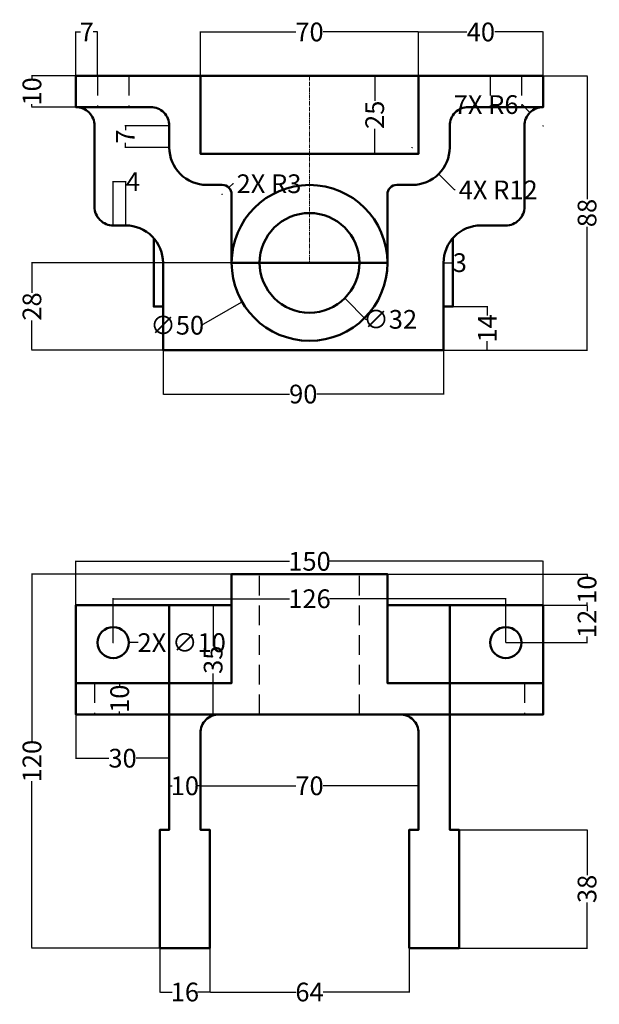
# Model space of a CAD drawing. Units: millimetres. Extents: x 17 to 203, y -197 to 119.
import ezdxf

# ---------------------------------------------------------------- set-up
doc = ezdxf.new("R2010")
doc.units = ezdxf.units.MM
doc.header["$MEASUREMENT"] = 0
doc.linetypes.add('CENTER', pattern=[2, 1.25, -0.25, 0.25, -0.25])
doc.linetypes.add('HIDDEN', pattern=[9.525, 6.35, -3.175])
for name, color, linetype, lineweight in [('M-CNTR', 4, 'CENTER', 18), ('M-CONS', 8, 'Continuous', 13), ('M-DIMS', 2, 'Continuous', 18), ('M-HIDN', 3, 'HIDDEN', 25), ('M-OUTL', 7, 'Continuous', 50)]:
    doc.layers.add(name, color=color, linetype=linetype, lineweight=lineweight)
doc.styles.get("Standard").update_dxf_attribs({"font": 'arial.ttf'})
doc.dimstyles.get("Standard").update_dxf_attribs({"dimtxt": 6, "dimasz": 0.18, "dimexe": 0.18, "dimexo": 0.0625, "dimgap": 0.09, "dimtad": 0, "dimtoh": 1, "dimdec": 0, "dimzin": 0, "dimdsep": 46, "dimtxsty": 'Standard', "dimcen": 0.09, "dimadec": 0, "dimazin": 0, "dimtfac": 1, "dimtdec": 0, "dimtofl": 0, "dimtmove": 0, "dimatfit": 3, "dimfxl": 1, "dimtolj": 1, "dimtzin": 0, "dimarcsym": 0})

# ---------------------------------------------------------------- blocks, each defined once
blk = doc.blocks.new('MOUNT-HOLE-D10')
blk.add_circle((0, 0), 5)
blk = doc.blocks.new('MOUNT-HOLE-D10-EDGE')
for p, q in [((-5, 10), (-5, 0)), ((5, 10), (5, 0))]:
    blk.add_line(p, q)
blk = doc.blocks.new('*D3')
at = {"layer": 'Defpoints', "color": 0, "transparency": 16777216}
for p in [(184.66, -55.03), (34.66, -69.11), (184.66, -69.11)]:
    blk.add_point(p, dxfattribs=at)
at = {"layer": 'M-DIMS', "color": 0, "lineweight": -2, "transparency": 16777216}
for p, q in [((34.66, -69.05), (34.66, -54.85)), ((34.84, -55.03), (103.23, -55.03)), ((184.48, -55.03), (116.08, -55.03)), ((184.66, -69.05), (184.66, -54.85))]:
    blk.add_line(p, q, dxfattribs=at)
at = {"layer": 'M-DIMS', "color": 0, "transparency": 16777216}
for points in [[(34.84, -55), (34.84, -55.06), (34.66, -55.03)], [(184.48, -55), (184.48, -55.06), (184.66, -55.03)]]:
    blk.add_solid(points, dxfattribs=at)
at = {"layer": 'M-DIMS', "color": 0, "transparency": 16777216, "insert": (109.66, -55.03), "char_height": 6, "attachment_point": 5}
blk.add_mtext('\\A1;150', dxfattribs=at)
blk = doc.blocks.new('*D4')
at = {"layer": 'Defpoints', "color": 0, "transparency": 16777216}
for p in [(41.66, 114.77), (34.66, 100.7), (41.66, 100.7)]:
    blk.add_point(p, dxfattribs=at)
at = {"layer": 'M-DIMS', "color": 0, "lineweight": -2, "transparency": 16777216}
for p, q in [((34.66, 100.76), (34.66, 114.95)), ((34.84, 114.77), (36.13, 114.77)), ((41.48, 114.77), (40.19, 114.77)), ((41.66, 100.76), (41.66, 114.95))]:
    blk.add_line(p, q, dxfattribs=at)
at = {"layer": 'M-DIMS', "color": 0, "transparency": 16777216}
for points in [[(34.84, 114.8), (34.84, 114.74), (34.66, 114.77)], [(41.48, 114.8), (41.48, 114.74), (41.66, 114.77)]]:
    blk.add_solid(points, dxfattribs=at)
at = {"layer": 'M-DIMS', "color": 0, "transparency": 16777216, "insert": (38.16, 114.77), "char_height": 6, "attachment_point": 5}
blk.add_mtext('\\A1;7', dxfattribs=at)
blk = doc.blocks.new('*D5')
at = {"layer": 'Defpoints', "color": 0, "transparency": 16777216}
for p in [(144.66, 114.77), (74.66, 100.7), (144.66, 100.7)]:
    blk.add_point(p, dxfattribs=at)
at = {"layer": 'M-DIMS', "color": 0, "lineweight": -2, "transparency": 16777216}
for p, q in [((74.66, 100.76), (74.66, 114.95)), ((74.84, 114.77), (105.31, 114.77)), ((144.48, 114.77), (114.01, 114.77)), ((144.66, 100.76), (144.66, 114.95))]:
    blk.add_line(p, q, dxfattribs=at)
at = {"layer": 'M-DIMS', "color": 0, "transparency": 16777216}
for points in [[(74.84, 114.8), (74.84, 114.74), (74.66, 114.77)], [(144.48, 114.8), (144.48, 114.74), (144.66, 114.77)]]:
    blk.add_solid(points, dxfattribs=at)
at = {"layer": 'M-DIMS', "color": 0, "transparency": 16777216, "insert": (109.66, 114.77), "char_height": 6, "attachment_point": 5}
blk.add_mtext('\\A1;70', dxfattribs=at)
blk = doc.blocks.new('*D6')
at = {"layer": 'Defpoints', "color": 0, "transparency": 16777216}
for p in [(184.66, 114.77), (144.66, 100.7), (184.66, 100.7)]:
    blk.add_point(p, dxfattribs=at)
at = {"layer": 'M-DIMS', "color": 0, "lineweight": -2, "transparency": 16777216}
for p, q in [((144.66, 100.76), (144.66, 114.95)), ((144.84, 114.77), (160.16, 114.77)), ((184.48, 114.77), (169.16, 114.77)), ((184.66, 100.76), (184.66, 114.95))]:
    blk.add_line(p, q, dxfattribs=at)
at = {"layer": 'M-DIMS', "color": 0, "transparency": 16777216}
for points in [[(144.84, 114.8), (144.84, 114.74), (144.66, 114.77)], [(184.48, 114.8), (184.48, 114.74), (184.66, 114.77)]]:
    blk.add_solid(points, dxfattribs=at)
at = {"layer": 'M-DIMS', "color": 0, "transparency": 16777216, "insert": (164.66, 114.77), "char_height": 6, "attachment_point": 5}
blk.add_mtext('\\A1;40', dxfattribs=at)
blk = doc.blocks.new('*D7')
at = {"layer": 'Defpoints', "color": 0, "transparency": 16777216}
for p in [(184.66, 100.7), (152.66, 12.7), (198.73, 12.7)]:
    blk.add_point(p, dxfattribs=at)
at = {"layer": 'M-DIMS', "color": 0, "lineweight": -2, "transparency": 16777216}
for p, q in [((184.72, 100.7), (198.91, 100.7)), ((198.73, 100.52), (198.73, 61.09)), ((198.73, 12.88), (198.73, 52.3)), ((152.72, 12.7), (198.91, 12.7))]:
    blk.add_line(p, q, dxfattribs=at)
at = {"layer": 'M-DIMS', "color": 0, "transparency": 16777216}
for points in [[(198.7, 100.52), (198.76, 100.52), (198.73, 100.7)], [(198.7, 12.88), (198.76, 12.88), (198.73, 12.7)]]:
    blk.add_solid(points, dxfattribs=at)
at = {"layer": 'M-DIMS', "color": 0, "transparency": 16777216, "insert": (198.73, 56.7), "char_height": 6, "attachment_point": 5, "rotation": 90}
blk.add_mtext('\\A1;88', dxfattribs=at)
blk = doc.blocks.new('*D8')
at = {"layer": 'Defpoints', "color": 0, "transparency": 16777216}
for p in [(34.66, 100.7), (20.58, 90.7), (34.66, 90.7)]:
    blk.add_point(p, dxfattribs=at)
at = {"layer": 'M-DIMS', "color": 0, "lineweight": -2, "transparency": 16777216}
for p, q in [((34.6, 100.7), (20.4, 100.7)), ((20.58, 100.52), (20.58, 99.79)), ((20.58, 90.88), (20.58, 91.6)), ((34.6, 90.7), (20.4, 90.7))]:
    blk.add_line(p, q, dxfattribs=at)
at = {"layer": 'M-DIMS', "color": 0, "transparency": 16777216}
for points in [[(20.55, 100.52), (20.61, 100.52), (20.58, 100.7)], [(20.55, 90.88), (20.61, 90.88), (20.58, 90.7)]]:
    blk.add_solid(points, dxfattribs=at)
at = {"layer": 'M-DIMS', "color": 0, "transparency": 16777216, "insert": (20.58, 95.7), "char_height": 6, "attachment_point": 5, "rotation": 90}
blk.add_mtext('\\A1;10', dxfattribs=at)
blk = doc.blocks.new('*D9')
at = {"layer": 'Defpoints', "color": 0, "transparency": 16777216}
for p in [(130.58, 100.7), (144.66, 100.7), (144.66, 75.7)]:
    blk.add_point(p, dxfattribs=at)
at = {"layer": 'M-DIMS', "color": 0, "lineweight": -2, "transparency": 16777216}
for p, q in [((144.6, 100.7), (130.4, 100.7)), ((130.58, 100.52), (130.58, 92.66)), ((130.58, 75.88), (130.58, 83.74)), ((144.6, 75.7), (130.4, 75.7))]:
    blk.add_line(p, q, dxfattribs=at)
at = {"layer": 'M-DIMS', "color": 0, "transparency": 16777216}
for points in [[(130.55, 100.52), (130.61, 100.52), (130.58, 100.7)], [(130.55, 75.88), (130.61, 75.88), (130.58, 75.7)]]:
    blk.add_solid(points, dxfattribs=at)
at = {"layer": 'M-DIMS', "color": 0, "transparency": 16777216, "insert": (130.58, 88.2), "char_height": 6, "attachment_point": 5, "rotation": 90}
blk.add_mtext('\\A1;25', dxfattribs=at)
blk = doc.blocks.new('*D10')
at = {"layer": 'Defpoints', "color": 0, "transparency": 16777216}
for p in [(20.58, 40.7), (84.66, 40.7), (62.66, 12.7)]:
    blk.add_point(p, dxfattribs=at)
at = {"layer": 'M-DIMS', "color": 0, "lineweight": -2, "transparency": 16777216}
for p, q in [((84.6, 40.7), (20.4, 40.7)), ((20.58, 40.52), (20.58, 31.14)), ((20.58, 12.88), (20.58, 22.25)), ((62.6, 12.7), (20.4, 12.7))]:
    blk.add_line(p, q, dxfattribs=at)
at = {"layer": 'M-DIMS', "color": 0, "transparency": 16777216}
for points in [[(20.55, 40.52), (20.61, 40.52), (20.58, 40.7)], [(20.55, 12.88), (20.61, 12.88), (20.58, 12.7)]]:
    blk.add_solid(points, dxfattribs=at)
at = {"layer": 'M-DIMS', "color": 0, "transparency": 16777216, "insert": (20.58, 26.7), "char_height": 6, "attachment_point": 5, "rotation": 90}
blk.add_mtext('\\A1;28', dxfattribs=at)
blk = doc.blocks.new('*D11')
at = {"layer": 'Defpoints', "color": 0, "transparency": 16777216}
for p in [(62.66, 12.7), (152.66, 12.7), (62.66, -1.38)]:
    blk.add_point(p, dxfattribs=at)
at = {"layer": 'M-DIMS', "color": 0, "lineweight": -2, "transparency": 16777216}
for p, q in [((62.66, 12.63), (62.66, -1.56)), ((152.66, 12.63), (152.66, -1.56)), ((62.84, -1.38), (103.28, -1.38)), ((152.48, -1.38), (112.04, -1.38))]:
    blk.add_line(p, q, dxfattribs=at)
at = {"layer": 'M-DIMS', "color": 0, "transparency": 16777216}
for points in [[(62.84, -1.35), (62.84, -1.41), (62.66, -1.38)], [(152.48, -1.35), (152.48, -1.41), (152.66, -1.38)]]:
    blk.add_solid(points, dxfattribs=at)
at = {"layer": 'M-DIMS', "color": 0, "transparency": 16777216, "insert": (107.66, -1.38), "char_height": 6, "attachment_point": 5}
blk.add_mtext('\\A1;90', dxfattribs=at)
blk = doc.blocks.new('*D12')
at = {"layer": 'Defpoints', "color": 0, "transparency": 16777216}
for p in [(152.66, 26.7), (152.66, 12.7), (166.73, 12.7)]:
    blk.add_point(p, dxfattribs=at)
at = {"layer": 'M-DIMS', "color": 0, "lineweight": -2, "transparency": 16777216}
for p, q in [((152.72, 26.7), (166.91, 26.7)), ((166.73, 26.52), (166.73, 23.79)), ((152.72, 12.7), (166.91, 12.7)), ((166.73, 12.88), (166.73, 15.6))]:
    blk.add_line(p, q, dxfattribs=at)
at = {"layer": 'M-DIMS', "color": 0, "transparency": 16777216}
for points in [[(166.7, 26.52), (166.76, 26.52), (166.73, 26.7)], [(166.7, 12.88), (166.76, 12.88), (166.73, 12.7)]]:
    blk.add_solid(points, dxfattribs=at)
at = {"layer": 'M-DIMS', "color": 0, "transparency": 16777216, "insert": (166.73, 19.7), "char_height": 6, "attachment_point": 5, "rotation": 90}
blk.add_mtext('\\A1;14', dxfattribs=at)
blk = doc.blocks.new('*D13')
at = {"layer": 'Defpoints', "color": 0, "transparency": 16777216}
for p in [(155.66, 40.77), (152.66, 26.7), (155.66, 26.7)]:
    blk.add_point(p, dxfattribs=at)
at = {"layer": 'M-DIMS', "color": 0, "lineweight": -2, "transparency": 16777216}
for p, q in [((152.66, 26.76), (152.66, 40.95)), ((152.84, 40.77), (155.48, 40.77)), ((155.66, 26.76), (155.66, 40.95)), ((155.66, 40.77), (155.84, 40.77))]:
    blk.add_line(p, q, dxfattribs=at)
at = {"layer": 'M-DIMS', "color": 0, "transparency": 16777216}
for points in [[(152.84, 40.8), (152.84, 40.74), (152.66, 40.77)], [(155.48, 40.8), (155.48, 40.74), (155.66, 40.77)]]:
    blk.add_solid(points, dxfattribs=at)
at = {"layer": 'M-DIMS', "color": 0, "transparency": 16777216, "insert": (157.89, 40.77), "char_height": 6, "attachment_point": 5}
blk.add_mtext('\\A1;3', dxfattribs=at)
blk = doc.blocks.new('*D14')
at = {"layer": 'Defpoints', "color": 0, "transparency": 16777216}
for p in [(50.66, 66.77), (46.66, 52.7), (50.66, 52.7)]:
    blk.add_point(p, dxfattribs=at)
at = {"layer": 'M-DIMS', "color": 0, "lineweight": -2, "transparency": 16777216}
for p, q in [((46.66, 52.76), (46.66, 66.95)), ((46.84, 66.77), (50.48, 66.77)), ((50.66, 52.76), (50.66, 66.95)), ((50.66, 66.77), (50.84, 66.77))]:
    blk.add_line(p, q, dxfattribs=at)
at = {"layer": 'M-DIMS', "color": 0, "transparency": 16777216}
for points in [[(46.84, 66.8), (46.84, 66.74), (46.66, 66.77)], [(50.48, 66.8), (50.48, 66.74), (50.66, 66.77)]]:
    blk.add_solid(points, dxfattribs=at)
at = {"layer": 'M-DIMS', "color": 0, "transparency": 16777216, "insert": (53, 66.77), "char_height": 6, "attachment_point": 5}
blk.add_mtext('\\A1;4', dxfattribs=at)
blk = doc.blocks.new('*D15')
at = {"layer": 'Defpoints', "color": 0, "transparency": 16777216}
for p in [(50.58, 84.7), (64.66, 84.7), (64.66, 77.7)]:
    blk.add_point(p, dxfattribs=at)
at = {"layer": 'M-DIMS', "color": 0, "lineweight": -2, "transparency": 16777216}
for p, q in [((64.6, 84.7), (50.4, 84.7)), ((50.58, 84.52), (50.58, 83.23)), ((50.58, 77.88), (50.58, 79.16)), ((64.6, 77.7), (50.4, 77.7))]:
    blk.add_line(p, q, dxfattribs=at)
at = {"layer": 'M-DIMS', "color": 0, "transparency": 16777216}
for points in [[(50.55, 84.52), (50.61, 84.52), (50.58, 84.7)], [(50.55, 77.88), (50.61, 77.88), (50.58, 77.7)]]:
    blk.add_solid(points, dxfattribs=at)
at = {"layer": 'M-DIMS', "color": 0, "transparency": 16777216, "insert": (50.58, 81.2), "char_height": 6, "attachment_point": 5, "rotation": 90}
blk.add_mtext('\\A1;7', dxfattribs=at)
blk = doc.blocks.new('*D16')
at = {"layer": 'Defpoints', "color": 0, "transparency": 16777216}
for p in [(84.66, -59.11), (20.58, -179.11), (61.66, -179.11)]:
    blk.add_point(p, dxfattribs=at)
at = {"layer": 'M-DIMS', "color": 0, "lineweight": -2, "transparency": 16777216}
for p, q in [((84.6, -59.11), (20.4, -59.11)), ((20.58, -59.29), (20.58, -112.68)), ((20.58, -178.93), (20.58, -125.54)), ((61.6, -179.11), (20.4, -179.11))]:
    blk.add_line(p, q, dxfattribs=at)
at = {"layer": 'M-DIMS', "color": 0, "transparency": 16777216}
for points in [[(20.55, -59.29), (20.61, -59.29), (20.58, -59.11)], [(20.55, -178.93), (20.61, -178.93), (20.58, -179.11)]]:
    blk.add_solid(points, dxfattribs=at)
at = {"layer": 'M-DIMS', "color": 0, "transparency": 16777216, "insert": (20.58, -119.11), "char_height": 6, "attachment_point": 5, "rotation": 90}
blk.add_mtext('\\A1;120', dxfattribs=at)
blk = doc.blocks.new('*D17')
at = {"layer": 'Defpoints', "color": 0, "transparency": 16777216}
for p in [(172.66, -67.03), (46.66, -81.11), (172.66, -81.11)]:
    blk.add_point(p, dxfattribs=at)
at = {"layer": 'M-DIMS', "color": 0, "lineweight": -2, "transparency": 16777216}
for p, q in [((46.66, -81.05), (46.66, -66.85)), ((46.84, -67.03), (103.22, -67.03)), ((172.48, -67.03), (116.09, -67.03)), ((172.66, -81.05), (172.66, -66.85))]:
    blk.add_line(p, q, dxfattribs=at)
at = {"layer": 'M-DIMS', "color": 0, "transparency": 16777216}
for points in [[(46.84, -67), (46.84, -67.06), (46.66, -67.03)], [(172.48, -67), (172.48, -67.06), (172.66, -67.03)]]:
    blk.add_solid(points, dxfattribs=at)
at = {"layer": 'M-DIMS', "color": 0, "transparency": 16777216, "insert": (109.66, -67.03), "char_height": 6, "attachment_point": 5}
blk.add_mtext('\\A1;126', dxfattribs=at)
blk = doc.blocks.new('*D18')
at = {"layer": 'Defpoints', "color": 0, "transparency": 16777216}
for p in [(184.66, -69.11), (172.66, -81.11), (198.73, -81.11)]:
    blk.add_point(p, dxfattribs=at)
at = {"layer": 'M-DIMS', "color": 0, "lineweight": -2, "transparency": 16777216}
for p, q in [((184.72, -69.11), (198.91, -69.11)), ((198.73, -69.29), (198.73, -71.04)), ((172.72, -81.11), (198.91, -81.11)), ((198.73, -80.93), (198.73, -79.18))]:
    blk.add_line(p, q, dxfattribs=at)
at = {"layer": 'M-DIMS', "color": 0, "transparency": 16777216}
for points in [[(198.7, -69.29), (198.76, -69.29), (198.73, -69.11)], [(198.7, -80.93), (198.76, -80.93), (198.73, -81.11)]]:
    blk.add_solid(points, dxfattribs=at)
at = {"layer": 'M-DIMS', "color": 0, "transparency": 16777216, "insert": (198.73, -75.11), "char_height": 6, "attachment_point": 5, "rotation": 90}
blk.add_mtext('\\A1;12', dxfattribs=at)
blk = doc.blocks.new('*D19')
at = {"layer": 'Defpoints', "color": 0, "transparency": 16777216}
for p in [(134.66, -59.11), (198.73, -59.11), (184.66, -69.11)]:
    blk.add_point(p, dxfattribs=at)
at = {"layer": 'M-DIMS', "color": 0, "lineweight": -2, "transparency": 16777216}
for p, q in [((134.72, -59.11), (198.91, -59.11)), ((198.73, -59.29), (198.73, -60.01)), ((184.72, -69.11), (198.91, -69.11)), ((198.73, -68.93), (198.73, -68.2))]:
    blk.add_line(p, q, dxfattribs=at)
at = {"layer": 'M-DIMS', "color": 0, "transparency": 16777216}
for points in [[(198.7, -59.29), (198.76, -59.29), (198.73, -59.11)], [(198.7, -68.93), (198.76, -68.93), (198.73, -69.11)]]:
    blk.add_solid(points, dxfattribs=at)
at = {"layer": 'M-DIMS', "color": 0, "transparency": 16777216, "insert": (198.73, -64.11), "char_height": 6, "attachment_point": 5, "rotation": 90}
blk.add_mtext('\\A1;10', dxfattribs=at)
blk = doc.blocks.new('*D20')
at = {"layer": 'Defpoints', "color": 0, "transparency": 16777216}
for p in [(64.66, -69.11), (64.66, -104.11), (78.73, -104.11)]:
    blk.add_point(p, dxfattribs=at)
at = {"layer": 'M-DIMS', "color": 0, "lineweight": -2, "transparency": 16777216}
for p, q in [((64.72, -69.11), (78.91, -69.11)), ((78.73, -69.29), (78.73, -82.2)), ((78.73, -103.93), (78.73, -91.02)), ((64.72, -104.11), (78.91, -104.11))]:
    blk.add_line(p, q, dxfattribs=at)
at = {"layer": 'M-DIMS', "color": 0, "transparency": 16777216}
for points in [[(78.7, -69.29), (78.76, -69.29), (78.73, -69.11)], [(78.7, -103.93), (78.76, -103.93), (78.73, -104.11)]]:
    blk.add_solid(points, dxfattribs=at)
at = {"layer": 'M-DIMS', "color": 0, "transparency": 16777216, "insert": (78.73, -86.61), "char_height": 6, "attachment_point": 5, "rotation": 90}
blk.add_mtext('\\A1;35', dxfattribs=at)
blk = doc.blocks.new('*D21')
at = {"layer": 'Defpoints', "color": 0, "transparency": 16777216}
for p in [(34.66, -94.11), (34.66, -104.11), (48.73, -104.11)]:
    blk.add_point(p, dxfattribs=at)
at = {"layer": 'M-DIMS', "color": 0, "lineweight": -2, "transparency": 16777216}
for p, q in [((34.72, -94.11), (48.91, -94.11)), ((48.73, -94.29), (48.73, -95.01)), ((34.72, -104.11), (48.91, -104.11)), ((48.73, -103.93), (48.73, -103.2))]:
    blk.add_line(p, q, dxfattribs=at)
at = {"layer": 'M-DIMS', "color": 0, "transparency": 16777216}
for points in [[(48.7, -94.29), (48.76, -94.29), (48.73, -94.11)], [(48.7, -103.93), (48.76, -103.93), (48.73, -104.11)]]:
    blk.add_solid(points, dxfattribs=at)
at = {"layer": 'M-DIMS', "color": 0, "transparency": 16777216, "insert": (48.73, -99.11), "char_height": 6, "attachment_point": 5, "rotation": 90}
blk.add_mtext('\\A1;10', dxfattribs=at)
blk = doc.blocks.new('*D22')
at = {"layer": 'Defpoints', "color": 0, "transparency": 16777216}
for p in [(34.66, -104.11), (64.66, -104.11), (34.66, -118.18)]:
    blk.add_point(p, dxfattribs=at)
at = {"layer": 'M-DIMS', "color": 0, "lineweight": -2, "transparency": 16777216}
for p, q in [((34.66, -104.17), (34.66, -118.36)), ((64.66, -104.17), (64.66, -118.36)), ((34.84, -118.18), (45.28, -118.18)), ((64.48, -118.18), (54.03, -118.18))]:
    blk.add_line(p, q, dxfattribs=at)
at = {"layer": 'M-DIMS', "color": 0, "transparency": 16777216}
for points in [[(34.84, -118.15), (34.84, -118.21), (34.66, -118.18)], [(64.48, -118.15), (64.48, -118.21), (64.66, -118.18)]]:
    blk.add_solid(points, dxfattribs=at)
at = {"layer": 'M-DIMS', "color": 0, "transparency": 16777216, "insert": (49.66, -118.18), "char_height": 6, "attachment_point": 5}
blk.add_mtext('\\A1;30', dxfattribs=at)
blk = doc.blocks.new('*D23')
at = {"layer": 'Defpoints', "color": 0, "transparency": 16777216}
for p in [(144.66, -127.03), (74.66, -141.11), (144.66, -141.11)]:
    blk.add_point(p, dxfattribs=at)
at = {"layer": 'M-DIMS', "color": 0, "lineweight": -2, "transparency": 16777216}
for p, q in [((74.66, -141.05), (74.66, -126.85)), ((74.84, -127.03), (105.31, -127.03)), ((144.48, -127.03), (114.01, -127.03)), ((144.66, -141.05), (144.66, -126.85))]:
    blk.add_line(p, q, dxfattribs=at)
at = {"layer": 'M-DIMS', "color": 0, "transparency": 16777216}
for points in [[(74.84, -127), (74.84, -127.06), (74.66, -127.03)], [(144.48, -127), (144.48, -127.06), (144.66, -127.03)]]:
    blk.add_solid(points, dxfattribs=at)
at = {"layer": 'M-DIMS', "color": 0, "transparency": 16777216, "insert": (109.66, -127.03), "char_height": 6, "attachment_point": 5}
blk.add_mtext('\\A1;70', dxfattribs=at)
blk = doc.blocks.new('*D24')
at = {"layer": 'Defpoints', "color": 0, "transparency": 16777216}
for p in [(74.66, -127.03), (64.66, -141.11), (74.66, -141.11)]:
    blk.add_point(p, dxfattribs=at)
at = {"layer": 'M-DIMS', "color": 0, "lineweight": -2, "transparency": 16777216}
for p, q in [((64.66, -141.05), (64.66, -126.85)), ((64.84, -127.03), (65.56, -127.03)), ((74.48, -127.03), (73.75, -127.03)), ((74.66, -141.05), (74.66, -126.85))]:
    blk.add_line(p, q, dxfattribs=at)
at = {"layer": 'M-DIMS', "color": 0, "transparency": 16777216}
for points in [[(64.84, -127), (64.84, -127.06), (64.66, -127.03)], [(74.48, -127), (74.48, -127.06), (74.66, -127.03)]]:
    blk.add_solid(points, dxfattribs=at)
at = {"layer": 'M-DIMS', "color": 0, "transparency": 16777216, "insert": (69.66, -127.03), "char_height": 6, "attachment_point": 5}
blk.add_mtext('\\A1;10', dxfattribs=at)
blk = doc.blocks.new('*D25')
at = {"layer": 'Defpoints', "color": 0, "transparency": 16777216}
for p in [(61.66, -179.11), (77.66, -179.11), (77.66, -193.18)]:
    blk.add_point(p, dxfattribs=at)
at = {"layer": 'M-DIMS', "color": 0, "lineweight": -2, "transparency": 16777216}
for p, q in [((61.66, -179.17), (61.66, -193.36)), ((77.66, -179.17), (77.66, -193.36)), ((61.84, -193.18), (65.56, -193.18)), ((77.48, -193.18), (73.76, -193.18))]:
    blk.add_line(p, q, dxfattribs=at)
at = {"layer": 'M-DIMS', "color": 0, "transparency": 16777216}
for points in [[(61.84, -193.15), (61.84, -193.21), (61.66, -193.18)], [(77.48, -193.15), (77.48, -193.21), (77.66, -193.18)]]:
    blk.add_solid(points, dxfattribs=at)
at = {"layer": 'M-DIMS', "color": 0, "transparency": 16777216, "insert": (69.66, -193.18), "char_height": 6, "attachment_point": 5}
blk.add_mtext('\\A1;16', dxfattribs=at)
blk = doc.blocks.new('*D26')
at = {"layer": 'Defpoints', "color": 0, "transparency": 16777216}
for p in [(77.66, -179.11), (141.66, -179.11), (141.66, -193.18)]:
    blk.add_point(p, dxfattribs=at)
at = {"layer": 'M-DIMS', "color": 0, "lineweight": -2, "transparency": 16777216}
for p, q in [((77.66, -179.17), (77.66, -193.36)), ((141.66, -179.17), (141.66, -193.36)), ((77.84, -193.18), (105.27, -193.18)), ((141.48, -193.18), (114.05, -193.18))]:
    blk.add_line(p, q, dxfattribs=at)
at = {"layer": 'M-DIMS', "color": 0, "transparency": 16777216}
for points in [[(77.84, -193.15), (77.84, -193.21), (77.66, -193.18)], [(141.48, -193.15), (141.48, -193.21), (141.66, -193.18)]]:
    blk.add_solid(points, dxfattribs=at)
at = {"layer": 'M-DIMS', "color": 0, "transparency": 16777216, "insert": (109.66, -193.18), "char_height": 6, "attachment_point": 5}
blk.add_mtext('\\A1;64', dxfattribs=at)
blk = doc.blocks.new('*D27')
at = {"layer": 'Defpoints', "color": 0, "transparency": 16777216}
for p in [(157.66, -141.11), (157.66, -179.11), (198.73, -179.11)]:
    blk.add_point(p, dxfattribs=at)
at = {"layer": 'M-DIMS', "color": 0, "lineweight": -2, "transparency": 16777216}
for p, q in [((157.72, -141.11), (198.91, -141.11)), ((198.73, -141.29), (198.73, -155.72)), ((198.73, -178.93), (198.73, -164.5)), ((157.72, -179.11), (198.91, -179.11))]:
    blk.add_line(p, q, dxfattribs=at)
at = {"layer": 'M-DIMS', "color": 0, "transparency": 16777216}
for points in [[(198.7, -141.29), (198.76, -141.29), (198.73, -141.11)], [(198.7, -178.93), (198.76, -178.93), (198.73, -179.11)]]:
    blk.add_solid(points, dxfattribs=at)
at = {"layer": 'M-DIMS', "color": 0, "transparency": 16777216, "insert": (198.73, -160.11), "char_height": 6, "attachment_point": 5, "rotation": 90}
blk.add_mtext('\\A1;38', dxfattribs=at)
blk = doc.blocks.new('*D28')
at = {"layer": 'Defpoints', "color": 0, "transparency": 16777216}
for p in [(98.34, 52.01), (120.97, 29.38)]:
    blk.add_point(p, dxfattribs=at)
at = {"layer": 'M-DIMS', "color": 0, "lineweight": -2, "transparency": 16777216}
for p, q in [((109.57, 40.7), (109.75, 40.7)), ((109.66, 40.61), (109.66, 40.79)), ((127.76, 22.59), (121.1, 29.26)), ((127.94, 22.59), (127.76, 22.59))]:
    blk.add_line(p, q, dxfattribs=at)
at = {"layer": 'M-DIMS', "color": 0, "transparency": 16777216}
blk.add_solid([(121.12, 29.28), (121.08, 29.23), (120.97, 29.38)], dxfattribs=at)
at = {"layer": 'M-DIMS', "color": 0, "transparency": 16777216, "insert": (135.56, 22.59), "char_height": 6, "attachment_point": 5}
blk.add_mtext('\\A1;∅32', dxfattribs=at)
blk = doc.blocks.new('*D29')
at = {"layer": 'Defpoints', "color": 0, "transparency": 16777216}
for p in [(131.31, 53.2), (88.01, 28.2)]:
    blk.add_point(p, dxfattribs=at)
at = {"layer": 'M-DIMS', "color": 0, "lineweight": -2, "transparency": 16777216}
for p, q in [((109.57, 40.7), (109.75, 40.7)), ((109.66, 40.61), (109.66, 40.79)), ((75.02, 20.7), (87.85, 28.11)), ((74.84, 20.7), (75.02, 20.7))]:
    blk.add_line(p, q, dxfattribs=at)
at = {"layer": 'M-DIMS', "color": 0, "transparency": 16777216}
blk.add_solid([(87.84, 28.13), (87.87, 28.08), (88.01, 28.2)], dxfattribs=at)
at = {"layer": 'M-DIMS', "color": 0, "transparency": 16777216, "insert": (67.2, 20.7), "char_height": 6, "attachment_point": 5}
blk.add_mtext('\\A1;∅50', dxfattribs=at)
blk = doc.blocks.new('*D30')
at = {"layer": 'Defpoints', "color": 0, "transparency": 16777216}
for p in [(142.66, 77.7), (151.14, 69.21)]:
    blk.add_point(p, dxfattribs=at)
at = {"layer": 'M-DIMS', "color": 0, "lineweight": -2, "transparency": 16777216}
for p, q in [((142.57, 77.7), (142.75, 77.7)), ((142.66, 77.61), (142.66, 77.79)), ((156.23, 64.12), (151.27, 69.08)), ((156.41, 64.12), (156.23, 64.12))]:
    blk.add_line(p, q, dxfattribs=at)
at = {"layer": 'M-DIMS', "color": 0, "transparency": 16777216}
blk.add_solid([(151.29, 69.1), (151.25, 69.06), (151.14, 69.21)], dxfattribs=at)
at = {"layer": 'M-DIMS', "color": 0, "transparency": 16777216, "insert": (170.21, 64.12), "char_height": 6, "attachment_point": 5}
blk.add_mtext('\\A1;4X R12', dxfattribs=at)
blk = doc.blocks.new('*D31')
at = {"layer": 'Defpoints', "color": 0, "transparency": 16777216}
for p in [(180.42, 88.94), (184.66, 84.7)]:
    blk.add_point(p, dxfattribs=at)
at = {"layer": 'M-DIMS', "color": 0, "lineweight": -2, "transparency": 16777216}
for p, q in [((177.69, 91.48), (177.87, 91.48)), ((177.87, 91.48), (180.29, 89.07)), ((184.57, 84.7), (184.75, 84.7)), ((184.66, 84.61), (184.66, 84.79))]:
    blk.add_line(p, q, dxfattribs=at)
at = {"layer": 'M-DIMS', "color": 0, "transparency": 16777216}
blk.add_solid([(180.31, 89.09), (180.27, 89.04), (180.42, 88.94)], dxfattribs=at)
at = {"layer": 'M-DIMS', "color": 0, "transparency": 16777216, "insert": (166.34, 91.48), "char_height": 6, "attachment_point": 5}
blk.add_mtext('\\A1;7X R6', dxfattribs=at)
blk = doc.blocks.new('*D32')
at = {"layer": 'Defpoints', "color": 0, "transparency": 16777216}
for p in [(83.78, 64.82), (81.66, 62.7)]:
    blk.add_point(p, dxfattribs=at)
at = {"layer": 'M-DIMS', "color": 0, "lineweight": -2, "transparency": 16777216}
for p, q in [((85.05, 66.09), (83.91, 64.94)), ((85.23, 66.09), (85.05, 66.09)), ((81.57, 62.7), (81.75, 62.7)), ((81.66, 62.61), (81.66, 62.79))]:
    blk.add_line(p, q, dxfattribs=at)
at = {"layer": 'M-DIMS', "color": 0, "transparency": 16777216}
blk.add_solid([(83.89, 64.97), (83.93, 64.92), (83.78, 64.82)], dxfattribs=at)
at = {"layer": 'M-DIMS', "color": 0, "transparency": 16777216, "insert": (96.66, 66.09), "char_height": 6, "attachment_point": 5}
blk.add_mtext('\\A1;2X R3', dxfattribs=at)
blk = doc.blocks.new('*D33')
at = {"layer": 'Defpoints', "color": 0, "transparency": 16777216}
for p in [(41.66, -81.11), (51.66, -81.11)]:
    blk.add_point(p, dxfattribs=at)
at = {"layer": 'M-DIMS', "color": 0, "lineweight": -2, "transparency": 16777216}
for p, q in [((46.57, -81.11), (46.75, -81.11)), ((46.66, -81.2), (46.66, -81.02)), ((54.66, -81.11), (51.84, -81.11))]:
    blk.add_line(p, q, dxfattribs=at)
at = {"layer": 'M-DIMS', "color": 0, "transparency": 16777216}
blk.add_solid([(51.84, -81.08), (51.84, -81.14), (51.66, -81.11)], dxfattribs=at)
at = {"layer": 'M-DIMS', "color": 0, "transparency": 16777216, "insert": (68.64, -81.11), "char_height": 6, "attachment_point": 5}
blk.add_mtext('\\A1;2X ∅10', dxfattribs=at)

msp = doc.modelspace()

# ---------------------------------------------------------------- linework, layer by layer
at = {"layer": 'M-CNTR'}
msp.add_line((109.66, 100.7), (109.66, 40.7), dxfattribs=at)
at = {"layer": 'M-CONS'}
for p, q in [((34.66, 90.7), (34.66, 90.7)), ((184.66, 90.7), (184.66, 90.7))]:
    msp.add_line(p, q, dxfattribs=at)
at = {"layer": 'M-HIDN'}
for p, q in [((93.66, -104.11), (93.66, -59.11)), ((125.66, -104.11), (125.66, -59.11)), ((40.66, -94.11), (40.66, -104.11)), ((178.66, -94.11), (178.66, -104.11))]:
    msp.add_line(p, q, dxfattribs=at)
at = {"layer": 'M-OUTL'}
for points in [[(74.66, 100.7), (34.66, 100.7), (34.66, 90.7)], [(144.66, 100.7), (144.66, 75.7), (74.66, 75.7), (74.66, 100.7), (144.66, 100.7), (184.66, 100.7), (184.66, 90.7)], [(62.66, 26.7), (59.66, 26.7), (59.66, 48.63)], [(152.66, 26.7), (155.66, 26.7), (155.66, 48.63)], [(80.66, -104.11), (34.66, -104.11), (34.66, -94.11), (84.66, -94.11), (84.66, -59.11), (134.66, -59.11), (134.66, -94.11), (184.66, -94.11), (184.66, -69.11), (134.66, -69.11)], [(34.66, -94.11), (34.66, -69.11), (84.66, -69.11)]]:
    msp.add_lwpolyline(points, dxfattribs=at)
msp.add_lwpolyline([(178.66, 58.7), (178.66, 84.7, -0.414214), (184.66, 90.7), (160.66, 90.7, 0.414214), (154.66, 84.7), (154.66, 77.7, -0.414214), (142.66, 65.7), (137.66, 65.7, 0.414214), (134.66, 62.7), (134.66, 40.7), (84.66, 40.7), (84.66, 62.7, 0.414214), (81.66, 65.7), (76.66, 65.7, -0.414214), (64.66, 77.7), (64.66, 84.7, 0.414214), (58.66, 90.7), (34.66, 90.7, -0.414214), (40.66, 84.7), (40.66, 58.7, 0.414214), (46.66, 52.7), (50.66, 52.7, -0.414214), (62.66, 40.7), (62.66, 12.7), (152.66, 12.7), (152.66, 40.7, -0.414214), (164.66, 52.7), (172.66, 52.7, 0.414214)], format="xyb", close=True, dxfattribs=at)
for points in [[(138.66, -104.11), (80.66, -104.11, 0.414214), (74.66, -110.11), (74.66, -114.11), (74.66, -141.11), (77.66, -141.11), (77.66, -160.11), (77.66, -179.11), (61.66, -179.11), (61.66, -160.11), (61.66, -141.11), (64.66, -141.11), (64.66, -114.11), (64.66, -104.11), (64.66, -69.11)], [(154.66, -69.11), (154.66, -104.11), (154.66, -114.11), (154.66, -141.11), (157.66, -141.11), (157.66, -179.11), (141.66, -179.11), (141.66, -141.11), (144.66, -141.11), (144.66, -114.11), (144.66, -110.11, 0.414214), (138.66, -104.11), (184.66, -104.11), (184.66, -94.11)]]:
    msp.add_lwpolyline(points, format="xyb", dxfattribs=at)
for radius in [25, 16]:
    msp.add_circle((109.66, 40.7), radius, dxfattribs=at)

# ---------------------------------------------------------------- block references
at = {"layer": 'M-HIDN'}
for p in [(46.66, 90.7), (172.66, 90.7)]:
    msp.add_blockref('MOUNT-HOLE-D10-EDGE', p, dxfattribs=at)
at = {"layer": 'M-OUTL'}
for p in [(46.66, -81.11), (172.66, -81.11)]:
    msp.add_blockref('MOUNT-HOLE-D10', p, dxfattribs=at)

# ---------------------------------------------------------------- dimensions: what is measured, and where the dimension line sits
at = {"layer": 'M-DIMS'}
for base, p1, p2, picture, middle in [((41.66, 114.77), (34.66, 100.7), (41.66, 100.7), '*D4', (38.16, 114.77)), ((144.66, 114.77), (74.66, 100.7), (144.66, 100.7), '*D5', (109.66, 114.77)), ((184.66, 114.77), (144.66, 100.7), (184.66, 100.7), '*D6', (164.66, 114.77)), ((50.66, 66.77), (46.66, 52.7), (50.66, 52.7), '*D14', (53, 66.77)), ((155.66, 40.77), (152.66, 26.7), (155.66, 26.7), '*D13', (157.89, 40.77)), ((184.66, -55.03), (34.66, -69.11), (184.66, -69.11), '*D3', (109.66, -55.03)), ((172.66, -67.03), (46.66, -81.11), (172.66, -81.11), '*D17', (109.66, -67.03)), ((74.66, -127.03), (64.66, -141.11), (74.66, -141.11), '*D24', (69.66, -127.03)), ((144.66, -127.03), (74.66, -141.11), (144.66, -141.11), '*D23', (109.66, -127.03)), ((77.66, -193.18), (61.66, -179.11), (77.66, -179.11), '*D25', (69.66, -193.18)), ((141.66, -193.18), (77.66, -179.11), (141.66, -179.11), '*D26', (109.66, -193.18))]:
    dim = msp.add_linear_dim(base=base, p1=p1, p2=p2, dimstyle='Standard', override={"dimdec": 0, "dimlfac": 1, "dimrnd": 0, "dimzin": 0, "dimdsep": 46, "dimlunit": 2}, dxfattribs=at)
    dim.commit()
    dim.dimension.update_dxf_attribs({"geometry": picture, "text_midpoint": middle})
for base, p1, p2, angle, picture, middle in [((20.58, 90.7), (34.66, 100.7), (34.66, 90.7), 90, '*D8', (20.58, 95.7)), ((130.58, 100.7), (144.66, 75.7), (144.66, 100.7), 90, '*D9', (130.58, 88.2)), ((198.73, 12.7), (184.66, 100.7), (152.66, 12.7), 90, '*D7', (198.73, 56.7)), ((50.58, 84.7), (64.66, 77.7), (64.66, 84.7), 90, '*D15', (50.58, 81.2)), ((20.58, 40.7), (62.66, 12.7), (84.66, 40.7), 90, '*D10', (20.58, 26.7)), ((166.73, 12.7), (152.66, 26.7), (152.66, 12.7), 270, '*D12', (166.73, 19.7)), ((62.66, -1.38), (152.66, 12.7), (62.66, 12.7), 180, '*D11', (107.66, -1.38)), ((20.58, -179.11), (84.66, -59.11), (61.66, -179.11), 90, '*D16', (20.58, -119.11)), ((198.73, -59.11), (184.66, -69.11), (134.66, -59.11), 90, '*D19', (198.73, -64.11)), ((78.73, -104.11), (64.66, -69.11), (64.66, -104.11), 270, '*D20', (78.73, -86.61)), ((198.73, -81.11), (184.66, -69.11), (172.66, -81.11), 90, '*D18', (198.73, -75.11)), ((48.73, -104.11), (34.66, -94.11), (34.66, -104.11), 270, '*D21', (48.73, -99.11)), ((34.66, -118.18), (64.66, -104.11), (34.66, -104.11), 180, '*D22', (49.66, -118.18)), ((198.73, -179.11), (157.66, -141.11), (157.66, -179.11), 90, '*D27', (198.73, -160.11))]:
    dim = msp.add_linear_dim(base=base, p1=p1, p2=p2, angle=angle, dimstyle='Standard', override={"dimdec": 0, "dimlfac": 1, "dimrnd": 0, "dimzin": 0, "dimdsep": 46, "dimlunit": 2}, dxfattribs=at)
    dim.commit()
    dim.dimension.update_dxf_attribs({"geometry": picture, "text_midpoint": middle})
for center, mpoint, text, picture, middle in [((184.66, 84.7), (180.42, 88.94), '7X <>', '*D31', (166.34, 91.48)), ((142.66, 77.7), (151.14, 69.21), '4X <>', '*D30', (170.21, 64.12)), ((81.66, 62.7), (83.78, 64.82), '2X <>', '*D32', (96.66, 66.09))]:
    dim = msp.add_radius_dim(center=center, mpoint=mpoint, text=text, dimstyle='Standard', override={"dimdec": 0, "dimlfac": 1, "dimrnd": 0, "dimzin": 0, "dimdsep": 46, "dimlunit": 2}, dxfattribs=at)
    dim.commit()
    dim.dimension.update_dxf_attribs({"geometry": picture, "text_midpoint": middle, "dimtype": 164})
for p1, p2, picture, middle in [((131.31, 53.2), (88.01, 28.2), '*D29', (67.2, 20.7)), ((98.34, 52.01), (120.97, 29.38), '*D28', (135.56, 22.59))]:
    dim = msp.add_diameter_dim_2p(p1=p1, p2=p2, dimstyle='Standard', override={"dimdec": 0, "dimlfac": 1, "dimrnd": 0, "dimzin": 0, "dimdsep": 46, "dimlunit": 2}, dxfattribs=at)
    dim.commit()
    dim.dimension.update_dxf_attribs({"geometry": picture, "text_midpoint": middle, "dimtype": 163})
dim = msp.add_diameter_dim_2p(p1=(41.66, -81.11), p2=(51.66, -81.11), text='2X <>', dimstyle='Standard', override={"dimdec": 0, "dimlfac": 1, "dimrnd": 0, "dimzin": 0, "dimdsep": 46, "dimlunit": 2}, dxfattribs=at)
dim.commit()
dim.dimension.update_dxf_attribs({"geometry": '*D33', "text_midpoint": (54.66, -81.11), "dimtype": 163})

doc.saveas('drawing.dxf')
